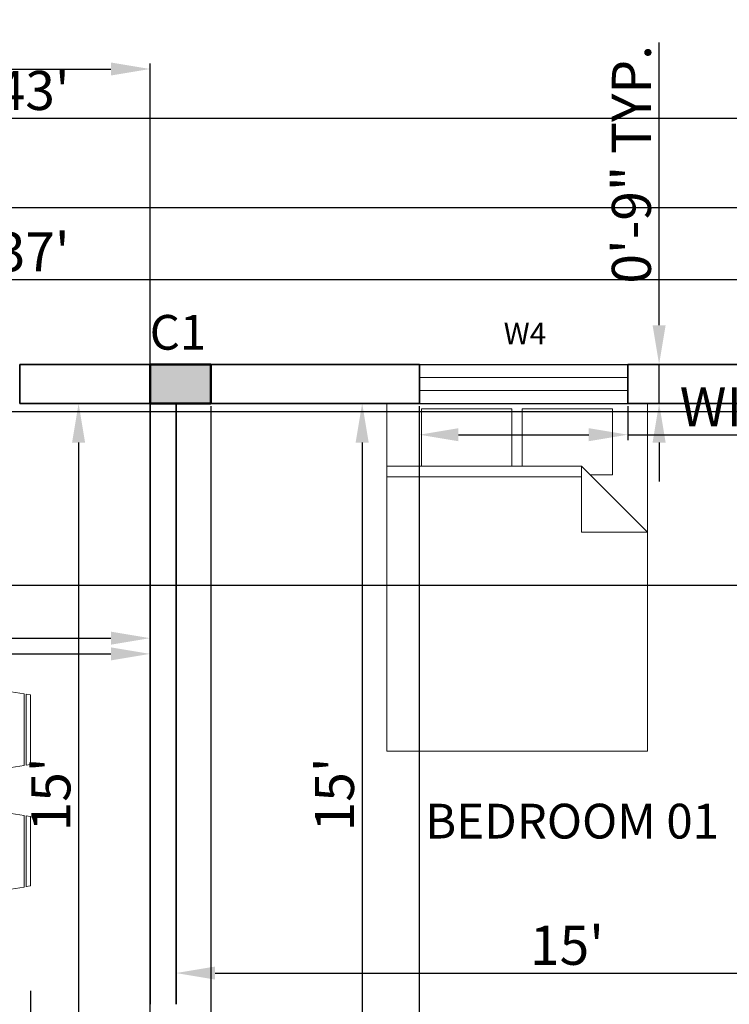
# Model space of a CAD drawing. Units: inches. Extents: x 2621 to 6190, y 513 to 1320.
# Tile 10 of 11: x 2997 to 3161, y 939 to 1165. Entities that reach past the tile are written whole.
import ezdxf

# ---------------------------------------------------------------- set-up
doc = ezdxf.new("R2010")
doc.units = ezdxf.units.IN
for name, color, linetype, lineweight in [('A-ANNO-DIMS', 5, 'Continuous', 18), ('A-ANNO-TEXT', 7, 'Continuous', 18), ('A-AREA-IDEN', 7, 'Continuous', 25), ('A-WALL', 7, 'Continuous', 35), ('C-PROP', 7, 'Continuous', 25), ('columns', 2, 'Continuous', 50), ('furniture', 30, 'Continuous', 18), ('S-COLS-IDEN', 2, 'Continuous', 25), ('S-COLS-PATT', 2, 'Continuous', 13), ('window', 172, 'Continuous', 18)]:
    doc.layers.add(name, color=color, linetype=linetype, lineweight=lineweight)
doc.styles.get("Standard").update_dxf_attribs({"font": 'arial.ttf'})
doc.dimstyles.new('ISO-25', dxfattribs={"dimtxt": 9, "dimasz": 9, "dimexe": 1.25, "dimexo": 0.625, "dimtad": 1, "dimlunit": 3, "dimtxsty": 'Standard', "dimcen": 2.5, "dimadec": 0, "dimazin": 0, "dimtfac": 1, "dimtmove": 0, "dimatfit": 3, "dimfxl": 1, "dimarcsym": 0})

# ---------------------------------------------------------------- blocks, each defined once
blk = doc.blocks.new('Dining Set - 36 x 72 in.')
for p, q in [((-22, 27.5), (-22.1562, 26.50042)), ((-22, 27.5), (-6, 27.5)), ((-5.8437, 26.49966), (-6, 27.5)), ((6, 27.5), (5.8438, 26.50042)), ((6, 27.5), (22, 27.5)), ((22.1563, 26.49966), (22, 27.5)), ((-22.2343, 26.00059), (-23.4847, 17.99762)), ((-22.2304, 26), (-5.7608, 26)), ((-5.8416, 26.5), (-22.1534, 26.5)), ((-4.5152, 17.99762), (-5.7655, 25.99926)), ((5.7657, 26.00059), (4.5153, 17.99762)), ((5.7696, 26), (22.2392, 26)), ((22.1584, 26.5), (5.8466, 26.5)), ((23.4848, 17.99762), (22.2345, 25.99926)), ((36, 18), (-36, 18)), ((-36, 18), (-36, -18)), ((36, -18), (36, 18)), ((-44.0006, 8.23428), (-35.9976, 9.48474)), ((44.0006, 8.23428), (35.9976, 9.48474)), ((-45.5, 8), (-44.5004, 8.15617)), ((-45.5, 8), (-45.5, -8)), ((-44.5, -8.15843), (-44.5, 8.15338)), ((-44, 8.23041), (-44, -8.23915)), ((44, 8.23041), (44, -8.23915)), ((44.5, -8.15843), (44.5, 8.15338)), ((45.5, 8), (44.5005, 8.15617)), ((45.5, 8), (45.5, -8)), ((-44.4997, -8.15631), (-45.5, -8)), ((-35.9976, -9.48476), (-43.9993, -8.2345)), ((35.9976, -9.48476), (43.9993, -8.2345)), ((44.4997, -8.15631), (45.5, -8)), ((-36, -18), (36, -18)), ((-22.2343, -26.0006), (-23.4847, -17.99762)), ((-4.5152, -17.99762), (-5.7655, -25.99928)), ((5.7657, -26.0006), (4.5153, -17.99762)), ((23.4848, -17.99762), (22.2345, -25.99928)), ((-22.2304, -26), (-5.7608, -26)), ((-22, -27.5), (-22.1562, -26.50044)), ((-5.8416, -26.5), (-22.1534, -26.5)), ((-5.8437, -26.49967), (-6, -27.5)), ((5.7696, -26), (22.2392, -26)), ((6, -27.5), (5.8438, -26.50044)), ((22.1584, -26.5), (5.8466, -26.5)), ((22.1563, -26.49967), (22, -27.5)), ((-22, -27.5), (-6, -27.5)), ((6, -27.5), (22, -27.5))]:
    blk.add_line(p, q)
for points in [[(-36, 15), (-31.1772, 14.97754), (-26.8079, 14.91406), (-22.8538, 14.81543), (-19.276, 14.6875), (-16.0362, 14.53613), (-13.0957, 14.36718), (-10.4159, 14.18652), (-7.9583, 14), (-5.6904, 13.81315), (-3.6035, 13.63021), (-1.6954, 13.45508), (0.0365, 13.29166), (1.5945, 13.14388), (2.9811, 13.01562), (4.1988, 12.9108), (5.25, 12.83333), (6.1393, 12.78613), (6.8802, 12.76823), (7.4883, 12.77767), (7.9792, 12.8125), (8.3685, 12.87077), (8.6719, 12.95052), (8.9049, 13.0498), (9.0833, 13.16666), (9.2205, 13.29899), (9.3216, 13.44401), (9.3895, 13.59879), (9.4271, 13.76041), (9.4373, 13.92594), (9.4232, 14.09245), (9.3875, 14.257), (9.3333, 14.41666), (9.2638, 14.56917), (9.1836, 14.71484), (9.0975, 14.85465), (9.0104, 14.98958), (8.9272, 15.1206), (8.8529, 15.2487), (8.7922, 15.37483), (8.75, 15.5), (8.7305, 15.62467), (8.7344, 15.74739), (8.7617, 15.86621), (8.8125, 15.97916), (8.8867, 16.08431), (8.9844, 16.17968), (9.1055, 16.26334), (9.25, 16.33333), (9.4189, 16.38802), (9.6172, 16.42708), (9.8506, 16.45052), (10.125, 16.45833), (10.4463, 16.45052), (10.8203, 16.42708), (11.2529, 16.38802), (11.75, 16.33333), (12.3184, 16.26318), (12.9694, 16.17838), (13.7151, 16.07991), (14.5677, 15.96875), (15.5395, 15.84586), (16.6426, 15.71224), (17.8893, 15.56884), (19.2917, 15.41666), (20.859, 15.25667), (22.5879, 15.08984), (24.4721, 14.91715), (26.5052, 14.73958), (28.6809, 14.5581), (30.9929, 14.3737), (33.4347, 14.18733), (36, 14)], [(-36, 10), (-28.9766, 10.14274), (-23.1725, 10.20442), (-18.4241, 10.19775), (-14.5677, 10.13541), (-11.4399, 10.03011), (-8.877, 9.89453), (-6.7154, 9.74137), (-4.7917, 9.58333), (-2.9698, 9.43082), (-1.2246, 9.28515), (0.4415, 9.14534), (2.026, 9.01041), (3.5266, 8.87939), (4.9408, 8.7513), (6.266, 8.62516), (7.5, 8.5), (8.6411, 8.37549), (9.6914, 8.2539), (10.6538, 8.13818), (11.5312, 8.03125), (12.3267, 7.93603), (13.043, 7.85547), (13.6831, 7.79248), (14.25, 7.75), (14.7471, 7.7303), (15.1797, 7.73307), (15.5537, 7.75732), (15.875, 7.80208), (16.1494, 7.86637), (16.3828, 7.94922), (16.5811, 8.04964), (16.75, 8.16666), (16.8944, 8.29915), (17.0143, 8.44531), (17.1089, 8.60319), (17.1771, 8.77083), (17.218, 8.94629), (17.2305, 9.1276), (17.2137, 9.31282), (17.1667, 9.5), (17.0895, 9.6875), (16.987, 9.875), (16.8649, 10.0625), (16.7292, 10.25), (16.5856, 10.4375), (16.4401, 10.625), (16.2985, 10.8125), (16.1667, 11), (16.05, 11.18733), (15.9518, 11.3737), (15.8752, 11.5581), (15.8229, 11.73958), (15.798, 11.91715), (15.8034, 12.08984), (15.842, 12.25667), (15.9167, 12.41666), (16.0295, 12.56836), (16.1784, 12.70833), (16.3605, 12.83268), (16.5729, 12.9375), (16.8127, 13.01888), (17.0768, 13.07291), (17.3625, 13.0957), (17.6667, 13.08333), (17.9894, 13.03312), (18.3418, 12.94726), (18.7382, 12.82918), (19.1927, 12.68229), (19.7195, 12.51001), (20.3327, 12.31575), (21.0465, 12.10294), (21.875, 11.875), (22.8357, 11.63354), (23.959, 11.37304), (25.2786, 11.08618), (26.8282, 10.76562), (28.6414, 10.40405), (30.752, 9.99414), (33.1936, 9.52856), (36, 9)], [(-36, 5.5), (-30.7157, 5.3348), (-26.069, 5.20963), (-21.9946, 5.11767), (-18.4271, 5.05208), (-15.3009, 5.00602), (-12.5508, 4.97265), (-10.1112, 4.94515), (-7.9167, 4.91666), (-5.909, 4.88167), (-4.0586, 4.83984), (-2.3429, 4.79215), (-0.7396, 4.73958), (0.7739, 4.6831), (2.22, 4.6237), (3.6213, 4.56233), (5, 4.5), (6.373, 4.43782), (7.7344, 4.3776), (9.0723, 4.32129), (10.375, 4.27083), (11.6309, 4.22819), (12.8281, 4.19531), (13.9551, 4.17415), (15, 4.16666), (15.954, 4.17448), (16.819, 4.19791), (17.6001, 4.23698), (18.3021, 4.29166), (18.9299, 4.36198), (19.4883, 4.44791), (19.9823, 4.54948), (20.4167, 4.66666), (20.7969, 4.79899), (21.1302, 4.94401), (21.4245, 5.09879), (21.6875, 5.26041), (21.9271, 5.42594), (22.1511, 5.59245), (22.3672, 5.757), (22.5834, 5.91666), (22.8065, 6.06868), (23.0404, 6.21093), (23.2879, 6.34147), (23.5521, 6.45833), (23.8358, 6.55957), (24.142, 6.64323), (24.4735, 6.70735), (24.8334, 6.75), (25.2235, 6.76969), (25.642, 6.76692), (26.0858, 6.74267), (26.5521, 6.69791), (27.0379, 6.63362), (27.5404, 6.55078), (28.0565, 6.45036), (28.5834, 6.33333), (29.1242, 6.19987), (29.7071, 6.04687), (30.3661, 5.87044), (31.1354, 5.66666), (32.0493, 5.43164), (33.142, 5.16146), (34.4475, 4.85221), (36, 4.5)], [(-36, -1), (-30.7915, -0.6591), (-26.0195, -0.38216), (-21.6519, -0.16284), (-17.6563, 0.00521), (-14.0005, 0.12833), (-10.6523, 0.21289), (-7.5796, 0.26522), (-4.75, 0.29166), (-2.134, 0.29793), (0.2878, 0.28711), (2.5317, 0.26163), (4.6146, 0.22396), (6.5529, 0.17651), (8.3633, 0.12174), (10.0623, 0.06209), (11.6667, 0), (13.1899, -0.06201), (14.6341, -0.1211), (15.9982, -0.17432), (17.2813, -0.21875), (18.4823, -0.25147), (19.6003, -0.26953), (20.6343, -0.27002), (21.5834, -0.25), (22.4481, -0.20768), (23.2357, -0.14584), (23.9549, -0.06836), (24.6146, 0.02083), (25.2235, 0.11784), (25.7904, 0.21875), (26.3241, 0.31966), (26.8334, 0.41666), (27.3265, 0.50618), (27.8099, 0.58593), (28.2894, 0.65397), (28.7709, 0.70833), (29.2601, 0.74707), (29.763, 0.76823), (30.2855, 0.76985), (30.8334, 0.75), (31.4088, 0.70784), (31.9994, 0.64713), (32.589, 0.57275), (33.1615, 0.48958), (33.7008, 0.4025), (34.1908, 0.3164), (34.6153, 0.23616), (34.9584, 0.16666), (35.2099, 0.11165), (35.3848, 0.07031), (35.504, 0.04069), (35.5886, 0.02083), (35.6594, 0.00879), (35.7377, 0.0026), (35.8442, 0.00032), (36, 0)], [(-36, -6.5), (-27.1843, -6.31267), (-20.084, -6.1263), (-14.469, -5.9419), (-10.1094, -5.76042), (-6.7752, -5.58285), (-4.2363, -5.41016), (-2.2629, -5.24333), (-0.625, -5.08334), (0.8708, -4.93099), (2.2715, -4.78646), (3.5872, -4.64974), (4.8281, -4.52084), (6.0046, -4.39974), (7.127, -4.28646), (8.2053, -4.18099), (9.25, -4.08334), (10.2705, -3.99382), (11.2734, -3.91407), (12.2647, -3.84603), (13.25, -3.79167), (14.2354, -3.75293), (15.2266, -3.73177), (16.2295, -3.73015), (17.25, -3.75), (18.2912, -3.79248), (19.3451, -3.85547), (20.4009, -3.93604), (21.4479, -4.03125), (22.4754, -4.13819), (23.4727, -4.25391), (24.4289, -4.37549), (25.3334, -4.5), (26.1785, -4.62492), (26.9694, -4.74935), (27.7145, -4.87281), (28.4219, -4.99479), (29.1, -5.11483), (29.7572, -5.23242), (30.4016, -5.34709), (31.0417, -5.45834), (31.6837, -5.56437), (32.3262, -5.65821), (32.9658, -5.73153), (33.599, -5.77604), (34.2224, -5.78345), (34.8327, -5.74545), (35.4264, -5.65373), (36, -5.5)], [(-36, -10), (-26.4022, -9.81299), (-18.4675, -9.62891), (-11.9839, -9.45069), (-6.7396, -9.28125), (-2.5226, -9.12354), (0.8789, -8.98047), (3.6769, -8.85498), (6.0833, -8.75), (8.2767, -8.66765), (10.3021, -8.60677), (12.1712, -8.56543), (13.8958, -8.54167), (15.4876, -8.53353), (16.9583, -8.53907), (18.3197, -8.55632), (19.5834, -8.58334), (20.7616, -8.61841), (21.8685, -8.66081), (22.9188, -8.71004), (23.9271, -8.76563), (24.9081, -8.82707), (25.8763, -8.89388), (26.8465, -8.96558), (27.8334, -9.04167), (28.8474, -9.12118), (29.8828, -9.20117), (30.93, -9.27824), (31.9792, -9.34896), (33.0205, -9.40991), (34.0443, -9.45768), (35.0407, -9.48885), (36, -9.5)], [(-36, -14.5), (-30.0881, -14.33513), (-25.0332, -14.21224), (-20.7312, -14.12647), (-17.0781, -14.07292), (-13.97, -14.04671), (-11.3027, -14.04297), (-8.9724, -14.05681), (-6.875, -14.08334), (-4.9224, -14.11833), (-3.0905, -14.16016), (-1.3709, -14.20785), (0.2448, -14.26042), (1.7647, -14.3169), (3.1973, -14.3763), (4.5507, -14.43767), (5.8333, -14.5), (7.0554, -14.5621), (8.235, -14.62175), (9.3922, -14.67652), (10.5469, -14.72396), (11.7192, -14.76164), (12.929, -14.78711), (14.1965, -14.79794), (15.5417, -14.79167), (16.9933, -14.76424), (18.6152, -14.70508), (20.4804, -14.60197), (22.6615, -14.44271), (25.2312, -14.21509), (28.2624, -13.9069), (31.8277, -13.50594), (36, -13)]]:
    blk.add_lwpolyline(points)
blk = doc.blocks.new('Bed - Queen')
for p, q in [((0, -80.00003), (0, 0)), ((0, 0), (59.99999, 0)), ((59.99999, 0), (59.99999, -80.00003)), ((7.99999, -1.2), (28.79998, -1.2)), ((7.99999, -14.4), (7.99999, -1.2)), ((28.79998, -1.2), (28.79998, -14.4)), ((31.19999, -1.2), (51.99999, -1.2)), ((31.19999, -14.4), (31.19999, -1.2)), ((51.99999, -1.2), (51.99999, -16.4)), ((0, -14.4), (44.8, -14.4)), ((59.99999, -29.6), (44.8, -14.4)), ((44.8, -14.4), (44.8, -29.6)), ((44.8, -16.8), (0, -16.8)), ((51.99999, -16.4), (46.79936, -16.4)), ((44.8, -29.6), (59.99999, -29.6)), ((59.99999, -80.00003), (0, -80.00003))]:
    blk.add_line(p, q)
blk = doc.blocks.new('*D20')
at = {"layer": 'A-ANNO-DIMS', "color": 0, "lineweight": -2, "transparency": 16777216}
for p, q in [((2913.38, 1018.55), (2913.38, 1020.48)), ((3027.38, 1018.55), (3027.38, 1020.48)), ((2922.38, 1019.23), (3018.38, 1019.23))]:
    blk.add_line(p, q, dxfattribs=at)
at = {"layer": 'A-ANNO-DIMS', "color": 0, "transparency": 16777216}
for points in [[(2922.38, 1020.73), (2922.38, 1017.73), (2913.38, 1019.23)], [(3018.38, 1020.73), (3018.38, 1017.73), (3027.38, 1019.23)]]:
    blk.add_solid(points, dxfattribs=at)
at = {"layer": 'Defpoints', "color": 0, "transparency": 16777216}
for p in [(2913.38, 1017.92), (3027.38, 1019.23), (3027.38, 1017.92)]:
    blk.add_point(p, dxfattribs=at)
at = {"layer": 'A-ANNO-DIMS', "color": 0, "transparency": 16777216, "insert": (2970.38, 1024.45), "char_height": 9, "attachment_point": 5}
blk.add_mtext('9\'-6"', dxfattribs=at)
blk = doc.blocks.new('*D21')
at = {"layer": 'A-ANNO-DIMS', "color": 0, "lineweight": -2, "transparency": 16777216}
for p, q in [((2913.38, 1022.82), (2913.38, 1024.1)), ((2922.38, 1022.85), (3018.38, 1022.85)), ((3027.38, 1022.82), (3027.38, 1024.1))]:
    blk.add_line(p, q, dxfattribs=at)
at = {"layer": 'A-ANNO-DIMS', "color": 0, "transparency": 16777216}
for points in [[(2922.38, 1024.35), (2922.38, 1021.35), (2913.38, 1022.85)], [(3018.38, 1024.35), (3018.38, 1021.35), (3027.38, 1022.85)]]:
    blk.add_solid(points, dxfattribs=at)
at = {"layer": 'Defpoints', "color": 0, "transparency": 16777216}
for p in [(3027.38, 1022.85), (2913.38, 1022.19), (3027.38, 1022.19)]:
    blk.add_point(p, dxfattribs=at)
at = {"layer": 'A-ANNO-DIMS', "color": 0, "transparency": 16777216, "insert": (2970.38, 1028.07), "char_height": 9, "attachment_point": 5}
blk.add_mtext('9\'-6"', dxfattribs=at)
blk = doc.blocks.new('*D22')
at = {"layer": 'A-ANNO-DIMS', "color": 0, "lineweight": -2, "transparency": 16777216}
for p, q in [((3026.76, 1076.89), (3009.69, 1076.89)), ((3010.94, 1067.89), (3010.94, 905.89)), ((3026.76, 896.89), (3009.69, 896.89))]:
    blk.add_line(p, q, dxfattribs=at)
at = {"layer": 'A-ANNO-DIMS', "color": 0, "transparency": 16777216}
for points in [[(3009.44, 1067.89), (3012.44, 1067.89), (3010.94, 1076.89)], [(3009.44, 905.89), (3012.44, 905.89), (3010.94, 896.89)]]:
    blk.add_solid(points, dxfattribs=at)
at = {"layer": 'Defpoints', "color": 0, "transparency": 16777216}
for p in [(3027.38, 1076.89), (3010.94, 896.89), (3027.38, 896.89)]:
    blk.add_point(p, dxfattribs=at)
at = {"layer": 'A-ANNO-DIMS', "color": 0, "transparency": 16777216, "insert": (3005.72, 986.89), "char_height": 9, "attachment_point": 5, "rotation": 90}
blk.add_mtext("15'", dxfattribs=at)
blk = doc.blocks.new('*D23')
at = {"layer": 'A-ANNO-DIMS', "color": 0, "lineweight": -2, "transparency": 16777216}
for p, q in [((3069.48, 1076.89), (3077.47, 1076.89)), ((3076.22, 1067.89), (3076.22, 905.89)), ((3069.48, 896.89), (3077.47, 896.89))]:
    blk.add_line(p, q, dxfattribs=at)
at = {"layer": 'A-ANNO-DIMS', "color": 0, "transparency": 16777216}
for points in [[(3074.72, 1067.89), (3077.72, 1067.89), (3076.22, 1076.89)], [(3074.72, 905.89), (3077.72, 905.89), (3076.22, 896.89)]]:
    blk.add_solid(points, dxfattribs=at)
at = {"layer": 'Defpoints', "color": 0, "transparency": 16777216}
for p in [(3068.85, 1076.89), (3068.85, 896.89), (3076.22, 896.89)]:
    blk.add_point(p, dxfattribs=at)
at = {"layer": 'A-ANNO-DIMS', "color": 0, "transparency": 16777216, "insert": (3071, 986.89), "char_height": 9, "attachment_point": 5, "rotation": 90}
blk.add_mtext("15'", dxfattribs=at)
blk = doc.blocks.new('*D24')
at = {"layer": 'A-ANNO-DIMS', "color": 0, "lineweight": -2, "transparency": 16777216}
for p, q in [((3033.38, 1015.01), (3033.38, 944.49)), ((3213.38, 1015.01), (3213.38, 944.49)), ((3042.38, 945.74), (3204.38, 945.74))]:
    blk.add_line(p, q, dxfattribs=at)
at = {"layer": 'A-ANNO-DIMS', "color": 0, "transparency": 16777216}
for points in [[(3042.38, 947.24), (3042.38, 944.24), (3033.38, 945.74)], [(3204.38, 947.24), (3204.38, 944.24), (3213.38, 945.74)]]:
    blk.add_solid(points, dxfattribs=at)
at = {"layer": 'Defpoints', "color": 0, "transparency": 16777216}
for p in [(3033.38, 1015.63), (3213.38, 1015.63), (3213.38, 945.74)]:
    blk.add_point(p, dxfattribs=at)
at = {"layer": 'A-ANNO-DIMS', "color": 0, "transparency": 16777216, "insert": (3123.38, 950.97), "char_height": 9, "attachment_point": 5}
blk.add_mtext("15'", dxfattribs=at)
blk = doc.blocks.new('*D36')
at = {"layer": 'A-ANNO-DIMS', "color": 0, "lineweight": -2, "transparency": 16777216}
for p, q in [((2778.38, 1086.51), (2778.38, 1106.64)), ((3222.38, 1086.51), (3222.38, 1106.64)), ((2787.38, 1105.39), (3213.38, 1105.39))]:
    blk.add_line(p, q, dxfattribs=at)
at = {"layer": 'A-ANNO-DIMS', "color": 0, "transparency": 16777216}
for points in [[(2787.38, 1106.89), (2787.38, 1103.89), (2778.38, 1105.39)], [(3213.38, 1106.89), (3213.38, 1103.89), (3222.38, 1105.39)]]:
    blk.add_solid(points, dxfattribs=at)
at = {"layer": 'Defpoints', "color": 0, "transparency": 16777216}
for p in [(3222.38, 1105.39), (2778.38, 1085.89), (3222.38, 1085.89)]:
    blk.add_point(p, dxfattribs=at)
at = {"layer": 'A-ANNO-DIMS', "color": 0, "transparency": 16777216, "insert": (3000.38, 1110.61), "char_height": 9, "attachment_point": 5}
blk.add_mtext("37'", dxfattribs=at)
blk = doc.blocks.new('*D38')
at = {"layer": 'A-ANNO-DIMS', "color": 0, "lineweight": -2, "transparency": 16777216}
for p, q in [((2742.38, 1122.51), (2742.38, 1143.81)), ((2751.38, 1142.56), (3249.38, 1142.56)), ((3258.38, 1122.51), (3258.38, 1143.81))]:
    blk.add_line(p, q, dxfattribs=at)
at = {"layer": 'A-ANNO-DIMS', "color": 0, "transparency": 16777216}
for points in [[(2751.38, 1144.06), (2751.38, 1141.06), (2742.38, 1142.56)], [(3249.38, 1144.06), (3249.38, 1141.06), (3258.38, 1142.56)]]:
    blk.add_solid(points, dxfattribs=at)
at = {"layer": 'Defpoints', "color": 0, "transparency": 16777216}
for p in [(3258.38, 1142.56), (2742.38, 1121.89), (3258.38, 1121.89)]:
    blk.add_point(p, dxfattribs=at)
at = {"layer": 'A-ANNO-DIMS', "color": 0, "transparency": 16777216, "insert": (3000.38, 1147.79), "char_height": 9, "attachment_point": 5}
blk.add_mtext("43'", dxfattribs=at)
blk = doc.blocks.new('WIN-48IN')
for p, q in [((48, 9), (0, 9)), ((0, 9), (0, 0)), ((48, 0), (48, 9)), ((0, 6), (48, 6)), ((0, 3), (48, 3)), ((0, 0), (48, 0))]:
    blk.add_line(p, q)
blk = doc.blocks.new('*D55')
at = {"layer": 'A-ANNO-DIMS', "color": 0, "lineweight": -2, "transparency": 16777216}
for p, q in [((3089.38, 1076.26), (3089.38, 1068.44)), ((3137.38, 1076.26), (3137.38, 1068.44)), ((3098.38, 1069.69), (3128.38, 1069.69)), ((3137.38, 1069.69), (3261.52, 1069.69))]:
    blk.add_line(p, q, dxfattribs=at)
at = {"layer": 'A-ANNO-DIMS', "color": 0, "transparency": 16777216}
for points in [[(3098.38, 1071.19), (3098.38, 1068.19), (3089.38, 1069.69)], [(3128.38, 1071.19), (3128.38, 1068.19), (3137.38, 1069.69)]]:
    blk.add_solid(points, dxfattribs=at)
at = {"layer": 'Defpoints', "color": 0, "transparency": 16777216}
for p in [(3089.38, 1076.89), (3137.38, 1076.89), (3137.38, 1069.69)]:
    blk.add_point(p, dxfattribs=at)
at = {"layer": 'A-ANNO-DIMS', "color": 0, "transparency": 16777216, "insert": (3203.95, 1074.97), "char_height": 9, "attachment_point": 5}
blk.add_mtext('WINDOW 4\'-0" TYP.', dxfattribs=at)
blk = doc.blocks.new('*D56')
at = {"layer": 'A-ANNO-DIMS', "color": 0, "lineweight": -2, "transparency": 16777216}
for p, q in [((3144.58, 1094.89), (3144.58, 1160)), ((3138.01, 1085.89), (3145.83, 1085.89)), ((3144.58, 1076.89), (3144.58, 1085.89)), ((3138.01, 1076.89), (3145.83, 1076.89)), ((3144.58, 1067.89), (3144.58, 1058.89))]:
    blk.add_line(p, q, dxfattribs=at)
at = {"layer": 'A-ANNO-DIMS', "color": 0, "transparency": 16777216}
for points in [[(3143.08, 1094.89), (3146.08, 1094.89), (3144.58, 1085.89)], [(3143.08, 1067.89), (3146.08, 1067.89), (3144.58, 1076.89)]]:
    blk.add_solid(points, dxfattribs=at)
at = {"layer": 'Defpoints', "color": 0, "transparency": 16777216}
for p in [(3137.38, 1085.89), (3144.58, 1085.89), (3137.38, 1076.89)]:
    blk.add_point(p, dxfattribs=at)
at = {"layer": 'A-ANNO-DIMS', "color": 0, "transparency": 16777216, "insert": (3139.36, 1131.94), "char_height": 9, "attachment_point": 5, "rotation": 90}
blk.add_mtext('0\'-9" TYP.', dxfattribs=at)
blk = doc.blocks.new('*D74')
at = {"layer": 'A-ANNO-DIMS', "color": 0, "lineweight": -2, "transparency": 16777216}
for p, q in [((2944.88, 941.67), (2944.88, 927.39)), ((2999.88, 941.67), (2999.88, 927.39)), ((2953.88, 928.64), (2990.88, 928.64))]:
    blk.add_line(p, q, dxfattribs=at)
at = {"layer": 'A-ANNO-DIMS', "color": 0, "transparency": 16777216}
for points in [[(2953.88, 930.14), (2953.88, 927.14), (2944.88, 928.64)], [(2990.88, 930.14), (2990.88, 927.14), (2999.88, 928.64)]]:
    blk.add_solid(points, dxfattribs=at)
at = {"layer": 'Defpoints', "color": 0, "transparency": 16777216}
for p in [(2944.88, 942.29), (2999.88, 942.29), (2999.88, 928.64)]:
    blk.add_point(p, dxfattribs=at)
at = {"layer": 'A-ANNO-DIMS', "color": 0, "transparency": 16777216, "insert": (2972.38, 933.77), "char_height": 9, "attachment_point": 5}
blk.add_mtext('4\'-7"', dxfattribs=at)
blk = doc.blocks.new('*D80')
at = {"layer": 'A-ANNO-DIMS', "color": 0, "lineweight": -2, "transparency": 16777216}
for p, q in [((2907.38, 1086.51), (2907.38, 1155.14)), ((2916.38, 1153.89), (3018.38, 1153.89)), ((3027.38, 1086.51), (3027.38, 1155.14))]:
    blk.add_line(p, q, dxfattribs=at)
at = {"layer": 'A-ANNO-DIMS', "color": 0, "transparency": 16777216}
for points in [[(2916.38, 1155.39), (2916.38, 1152.39), (2907.38, 1153.89)], [(3018.38, 1155.39), (3018.38, 1152.39), (3027.38, 1153.89)]]:
    blk.add_solid(points, dxfattribs=at)
at = {"layer": 'Defpoints', "color": 0, "transparency": 16777216}
for p in [(3027.38, 1153.89), (2907.38, 1085.89), (3027.38, 1085.89)]:
    blk.add_point(p, dxfattribs=at)
at = {"layer": 'A-ANNO-DIMS', "color": 0, "transparency": 16777216, "insert": (2967.38, 1159.11), "char_height": 9, "attachment_point": 5}
blk.add_mtext('10\'-0"', dxfattribs=at)
blk = doc.blocks.new('*D83')
at = {"layer": 'A-ANNO-DIMS', "color": 0, "lineweight": -2, "transparency": 16777216}
for p, q in [((3028.01, 1085.89), (3291.63, 1085.89)), ((3290.38, 906.39), (3290.38, 1076.89)), ((3028.01, 897.39), (3291.63, 897.39))]:
    blk.add_line(p, q, dxfattribs=at)
at = {"layer": 'A-ANNO-DIMS', "color": 0, "transparency": 16777216}
for points in [[(3288.88, 1076.89), (3291.88, 1076.89), (3290.38, 1085.89)], [(3288.88, 906.39), (3291.88, 906.39), (3290.38, 897.39)]]:
    blk.add_solid(points, dxfattribs=at)
at = {"layer": 'Defpoints', "color": 0, "transparency": 16777216}
for p in [(3027.38, 1085.89), (3290.38, 1085.89), (3027.38, 897.39)]:
    blk.add_point(p, dxfattribs=at)
at = {"layer": 'A-ANNO-DIMS', "color": 0, "transparency": 16777216, "insert": (3285.1, 991.64), "char_height": 9, "attachment_point": 5, "rotation": 90}
blk.add_mtext('15\'-8 1/2"', dxfattribs=at)
blk = doc.blocks.new('*D88')
at = {"layer": 'A-ANNO-DIMS', "color": 0, "lineweight": -2, "transparency": 16777216}
for p, q in [((2910.22, 898.87), (2910.22, 1155.14)), ((2919.22, 1153.89), (3018.38, 1153.89)), ((3027.38, 898.01), (3027.38, 1155.14))]:
    blk.add_line(p, q, dxfattribs=at)
at = {"layer": 'A-ANNO-DIMS', "color": 0, "transparency": 16777216}
for points in [[(2919.22, 1155.39), (2919.22, 1152.39), (2910.22, 1153.89)], [(3018.38, 1155.39), (3018.38, 1152.39), (3027.38, 1153.89)]]:
    blk.add_solid(points, dxfattribs=at)
at = {"layer": 'Defpoints', "color": 0, "transparency": 16777216}
for p in [(3027.38, 1153.89), (2910.22, 898.24), (3027.38, 897.39)]:
    blk.add_point(p, dxfattribs=at)
at = {"layer": 'A-ANNO-DIMS', "color": 0, "transparency": 16777216, "insert": (2968.8, 1159.11), "char_height": 9, "attachment_point": 5}
blk.add_mtext('9\'-9"', dxfattribs=at)
blk = doc.blocks.new('*D102')
at = {"layer": 'A-ANNO-DIMS', "color": 0, "lineweight": -2, "transparency": 16777216}
for p, q in [((2915.57, 1054.4), (2915.57, 519.64)), ((2942.88, 1054.4), (2942.88, 519.64)), ((2924.57, 520.89), (2933.88, 520.89)), ((2942.88, 520.89), (2998.18, 520.89))]:
    blk.add_line(p, q, dxfattribs=at)
at = {"layer": 'A-ANNO-DIMS', "color": 0, "transparency": 16777216}
for points in [[(2924.57, 522.39), (2924.57, 519.39), (2915.57, 520.89)], [(2933.88, 522.39), (2933.88, 519.39), (2942.88, 520.89)]]:
    blk.add_solid(points, dxfattribs=at)
at = {"layer": 'Defpoints', "color": 0, "transparency": 16777216}
for p in [(2915.57, 1055.03), (2942.88, 1055.03), (2942.88, 520.89)]:
    blk.add_point(p, dxfattribs=at)
at = {"layer": 'A-ANNO-DIMS', "color": 0, "transparency": 16777216, "insert": (2975.03, 526.17), "char_height": 9, "attachment_point": 5}
blk.add_mtext('2\'-3 1/2"', dxfattribs=at)
blk = doc.blocks.new('*D103')
at = {"layer": 'A-ANNO-DIMS', "color": 0, "lineweight": -2, "transparency": 16777216}
for p, q in [((2929.85, 1075), (3291.63, 1075)), ((3290.38, 1044.05), (3290.38, 1066)), ((2929.85, 1035.05), (3291.63, 1035.05))]:
    blk.add_line(p, q, dxfattribs=at)
at = {"layer": 'A-ANNO-DIMS', "color": 0, "transparency": 16777216}
for points in [[(3288.88, 1066), (3291.88, 1066), (3290.38, 1075)], [(3288.88, 1044.05), (3291.88, 1044.05), (3290.38, 1035.05)]]:
    blk.add_solid(points, dxfattribs=at)
at = {"layer": 'Defpoints', "color": 0, "transparency": 16777216}
for p in [(2929.23, 1075), (3290.38, 1075), (2929.23, 1035.05)]:
    blk.add_point(p, dxfattribs=at)
at = {"layer": 'A-ANNO-DIMS', "color": 0, "transparency": 16777216, "insert": (3285.16, 1055.03), "char_height": 9, "attachment_point": 5, "rotation": 90}
blk.add_mtext('3\'-4"', dxfattribs=at)
blk = doc.blocks.new('*D107')
at = {"layer": 'A-ANNO-DIMS', "color": 0, "lineweight": -2, "transparency": 16777216}
for p, q in [((3041.38, 1076.26), (3041.38, 519.64)), ((3089.38, 1076.26), (3089.38, 519.64)), ((3050.38, 520.89), (3080.38, 520.89))]:
    blk.add_line(p, q, dxfattribs=at)
at = {"layer": 'A-ANNO-DIMS', "color": 0, "transparency": 16777216}
for points in [[(3050.38, 522.39), (3050.38, 519.39), (3041.38, 520.89)], [(3080.38, 522.39), (3080.38, 519.39), (3089.38, 520.89)]]:
    blk.add_solid(points, dxfattribs=at)
at = {"layer": 'Defpoints', "color": 0, "transparency": 16777216}
for p in [(3041.38, 1076.89), (3089.38, 1076.89), (3089.38, 520.89)]:
    blk.add_point(p, dxfattribs=at)
at = {"layer": 'A-ANNO-DIMS', "color": 0, "transparency": 16777216, "insert": (3065.38, 526.11), "char_height": 9, "attachment_point": 5}
blk.add_mtext('4\'-0"', dxfattribs=at)

msp = doc.modelspace()

# ---------------------------------------------------------------- hatches: boundary and pattern name
at = {"layer": 'S-COLS-PATT'}
h = msp.add_hatch(color=256, dxfattribs=at)
h.dxf.hatch_style = 1
h.paths.add_polyline_path([(2787.381, 1085.89), (2778.381, 1085.89), (2778.381, 1071.89), (2787.381, 1071.89)])
h.paths.add_polyline_path([(3222.381, 1085.89), (3208.381, 1085.89), (3208.381, 1076.89), (3222.381, 1076.89)])
h.paths.add_polyline_path([(3041.381, 1085.89), (3027.381, 1085.89), (3027.381, 1076.89), (3041.381, 1076.89)])
h.paths.add_polyline_path([(2916.381, 1085.89), (2907.381, 1085.89), (2907.381, 1076.89), (2916.381, 1076.89)])
h.paths.add_polyline_path([(2916.381, 1076.89), (2913.381, 1076.89), (2913.381, 1071.89), (2916.381, 1071.89)])
h.paths.add_polyline_path([(2913.381, 1076.89), (2907.381, 1076.89), (2907.381, 1071.89), (2913.381, 1071.89)])
h.paths.add_polyline_path([(2787.381, 896.89), (2778.381, 896.89), (2778.381, 882.89), (2787.381, 882.89)])
h.paths.add_polyline_path([(2924.221, 898.241), (2910.221, 898.241), (2910.221, 889.241), (2924.221, 889.241)])
h.paths.add_polyline_path([(3036.381, 896.89), (3033.381, 896.89), (3027.381, 897.385), (3027.381, 883.385), (3033.381, 883.385), (3033.381, 890.89), (3036.381, 890.89)])
h.paths.add_polyline_path([(3036.381, 890.89), (3033.381, 890.89), (3033.381, 883.385), (3036.381, 883.385)], flags=17)
h.paths.add_polyline_path([(3222.381, 897.745), (3213.381, 897.745), (3213.381, 883.745), (3222.381, 883.745)])
h.paths.add_polyline_path([(3222.381, 710.89), (3208.381, 710.89), (3208.381, 701.89), (3222.381, 701.89)])
h.paths.add_polyline_path([(3039.318, 710.89), (3021.318, 710.89), (3021.318, 701.89), (3039.318, 701.89)])
h.paths.add_polyline_path([(2796.381, 710.89), (2778.381, 710.89), (2778.381, 701.89), (2796.381, 701.89)])

# ---------------------------------------------------------------- linework, layer by layer
at = {"layer": 'A-WALL'}
for p, q in [((2997.381, 1085.89), (2997.381, 1076.89)), ((3089.381, 1085.89), (2997.381, 1085.89)), ((3089.381, 1085.89), (3089.381, 1076.89)), ((3222.381, 1085.89), (3137.381, 1085.89)), ((3137.381, 1085.89), (3137.381, 1076.89)), ((3089.381, 1076.89), (2997.381, 1076.89)), ((3027.381, 1076.89), (3027.381, 938.548)), ((3033.381, 1076.89), (3033.381, 938.548)), ((3213.381, 1076.89), (3137.381, 1076.89))]:
    msp.add_line(p, q, dxfattribs=at)
at = {"layer": 'C-PROP'}
msp.add_lwpolyline([(3258.381, 552.89), (3258.381, 1121.89), (2742.381, 1121.89), (2718.381, 552.89)], close=True, dxfattribs=at)
at = {"layer": 'columns'}
msp.add_lwpolyline([(3027.381, 1076.89), (3027.381, 1085.89), (3041.381, 1085.89), (3041.381, 1076.89)], close=True, dxfattribs=at)

# ---------------------------------------------------------------- block references
at = {"layer": 'furniture'}
msp.add_blockref('Bed - Queen', (3081.881, 1076.818), dxfattribs=at)
at = {"layer": 'furniture', "rotation": 270}
msp.add_blockref('Dining Set - 36 x 72 in.', (2972.381, 987.791), dxfattribs=at)
at = {"layer": 'window'}
msp.add_blockref('WIN-48IN', (3089.381, 1076.89), dxfattribs=at)

# ---------------------------------------------------------------- texts
at = {"layer": 'A-ANNO-TEXT', "insert": (3108.802, 1095.476), "char_height": 5, "attachment_point": 1}
msp.add_mtext_dynamic_manual_height_columns('W4', width=21.64382, gutter_width=12.5, heights=[0], dxfattribs=at)
at = {"layer": 'A-AREA-IDEN', "insert": (3090.702, 984.722), "char_height": 8, "attachment_point": 1}
msp.add_mtext_dynamic_manual_height_columns('BEDROOM 01', width=78.46141, gutter_width=12.5, heights=[0], dxfattribs=at)
at = {"layer": 'S-COLS-IDEN', "insert": (3027.305, 1097.27), "char_height": 8, "attachment_point": 1}
msp.add_mtext_dynamic_manual_height_columns('C1', width=53.01391, gutter_width=12.5, heights=[0], dxfattribs=at)

# ---------------------------------------------------------------- dimensions: what is measured, and where the dimension line sits
at = {"layer": 'A-ANNO-DIMS'}
for base, p1, p2, override, picture, middle in [((3027.381, 1153.89), (2907.381, 1085.89), (3027.381, 1085.89), {"dimdec": 1, "dimlfac": 1, "dimrnd": 0, "dimzin": 1, "dimdsep": 46, "dimlunit": 4, "dimfrac": 2}, '*D80', (2967.381, 1159.11)), ((3027.381, 1153.89), (2910.221, 898.241), (3027.381, 897.385), {"dimdec": 1, "dimlfac": 1, "dimrnd": 0, "dimzin": 1, "dimdsep": 46, "dimlunit": 4, "dimfrac": 2}, '*D88', (2968.801, 1159.11)), ((3258.381, 1142.564), (2742.381, 1121.89), (3258.381, 1121.89), {"dimclrd": 0, "dimclre": 0, "dimclrt": 0}, '*D38', (3000.381, 1147.788)), ((3222.381, 1105.387), (2778.381, 1085.89), (3222.381, 1085.89), {"dimclrd": 0, "dimclre": 0, "dimclrt": 0}, '*D36', (3000.381, 1110.61)), ((3089.381, 520.89), (3041.381, 1076.89), (3089.381, 1076.89), {"dimdec": 1, "dimlfac": 1, "dimrnd": 0, "dimzin": 1, "dimdsep": 46, "dimlunit": 4, "dimfrac": 2}, '*D107', (3065.381, 526.11)), ((2942.877, 520.89), (2915.573, 1055.025), (2942.877, 1055.025), {"dimdec": 1, "dimlfac": 1, "dimrnd": 0, "dimzin": 1, "dimdsep": 46, "dimlunit": 4, "dimfrac": 2}, '*D102', (2975.027, 526.171)), ((3027.381, 1022.85), (2913.381, 1022.192), (3027.381, 1022.192), {"dimclrd": 0, "dimclre": 0, "dimclrt": 0}, '*D21', (2970.381, 1028.07)), ((3027.381, 1019.235), (2913.381, 1017.92), (3027.381, 1017.92), {"dimclrd": 0, "dimclre": 0, "dimclrt": 0}, '*D20', (2970.381, 1024.455)), ((3213.381, 945.745), (3033.381, 1015.632), (3213.381, 1015.632), {"dimclrd": 0, "dimclre": 0, "dimclrt": 0}, '*D24', (3123.381, 950.965)), ((2999.881, 928.641), (2944.881, 942.291), (2999.881, 942.291), {"dimdec": 1, "dimlfac": 1, "dimrnd": 0, "dimzin": 1, "dimdsep": 46, "dimlunit": 4, "dimfrac": 2}, '*D74', (2972.381, 933.766))]:
    dim = msp.add_linear_dim(base=base, p1=p1, p2=p2, dimstyle='ISO-25', override=override, dxfattribs=at)
    dim.commit()
    dim.dimension.update_dxf_attribs({"geometry": picture, "text_midpoint": middle})
dim = msp.add_linear_dim(base=(3144.581, 1085.89), p1=(3137.381, 1076.89), p2=(3137.381, 1085.89), angle=90, text='<> TYP.', dimstyle='ISO-25', override={"dimdec": 1, "dimlfac": 1, "dimrnd": 0, "dimzin": 1, "dimdsep": 46, "dimlunit": 4, "dimfrac": 2}, dxfattribs=at)
dim.commit()
dim.dimension.update_dxf_attribs({"geometry": '*D56', "text_midpoint": (3139.361, 1131.944)})
dim = msp.add_linear_dim(base=(3137.381, 1069.69), p1=(3089.381, 1076.89), p2=(3137.381, 1076.89), text='WINDOW <> TYP.', dimstyle='ISO-25', override={"dimdec": 1, "dimlfac": 1, "dimrnd": 0, "dimzin": 1, "dimdsep": 46, "dimlunit": 4, "dimfrac": 2}, dxfattribs=at)
dim.commit()
dim.dimension.update_dxf_attribs({"geometry": '*D55', "text_midpoint": (3203.95, 1074.971)})
for base, p1, p2, override, picture, middle in [((3290.381, 1085.89), (3027.381, 897.385), (3027.381, 1085.89), {"dimdec": 1, "dimlfac": 1, "dimrnd": 0, "dimzin": 1, "dimdsep": 46, "dimlunit": 4, "dimfrac": 2}, '*D83', (3285.103, 991.637)), ((3010.942, 896.89), (3027.381, 1076.89), (3027.381, 896.89), {"dimclrd": 0, "dimclre": 0, "dimclrt": 0}, '*D22', (3005.722, 986.89)), ((3076.22, 896.89), (3068.85, 1076.89), (3068.85, 896.89), {"dimclrd": 0, "dimclre": 0, "dimclrt": 0}, '*D23', (3071, 986.89)), ((3290.381, 1075.001), (2929.225, 1035.049), (2929.225, 1075.001), {"dimdec": 1, "dimlfac": 1, "dimrnd": 0, "dimzin": 1, "dimdsep": 46, "dimlunit": 4, "dimfrac": 2}, '*D103', (3285.158, 1055.025))]:
    dim = msp.add_linear_dim(base=base, p1=p1, p2=p2, angle=90, dimstyle='ISO-25', override=override, dxfattribs=at)
    dim.commit()
    dim.dimension.update_dxf_attribs({"geometry": picture, "text_midpoint": middle})

doc.saveas('drawing.dxf')
